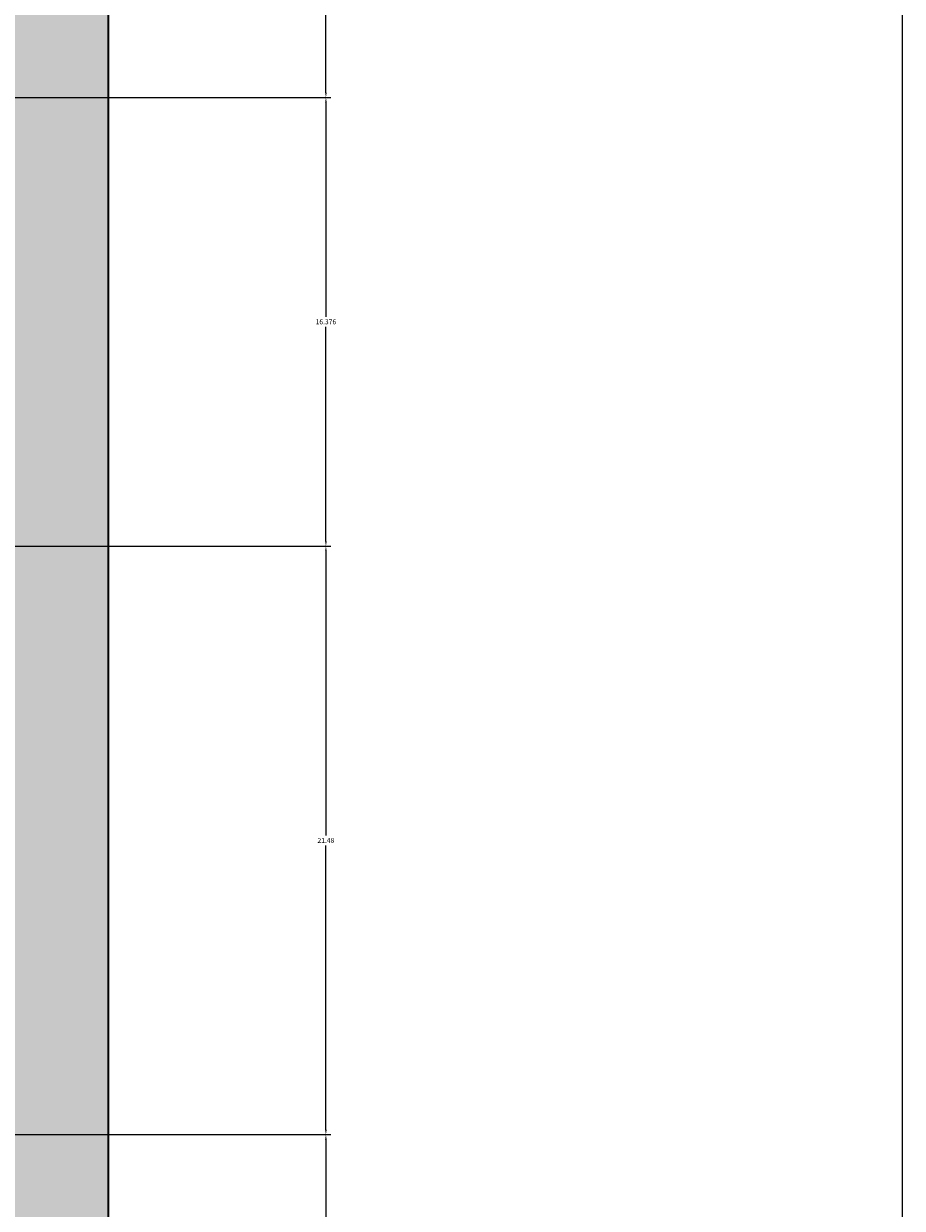
# Model space of a CAD drawing. Units: inches. Extents: x 4508 to 4723, y 847 to 1020.
# Tile 31 of 32: x 4691 to 4723, y 933 to 977. Entities that reach past the tile are written whole.
import ezdxf

# ---------------------------------------------------------------- set-up
doc = ezdxf.new("R2010")
doc.units = ezdxf.units.IN
for name, color, linetype, lineweight in [('A-ANNO-DIMS', 2, 'Continuous', 18), ('A-ANNO-TTLB', 7, 'Continuous', 25), ('A-WALL', 7, 'Continuous', 35), ('A-WALL-PATT', 254, 'Continuous', 13)]:
    doc.layers.add(name, color=color, linetype=linetype, lineweight=lineweight)
doc.styles.get("Standard").update_dxf_attribs({"font": 'arial.ttf'})
doc.dimstyles.get("Standard").update_dxf_attribs({"dimtxt": 0.18, "dimasz": 0.18, "dimexe": 0.18, "dimexo": 0.0625, "dimgap": 0.09, "dimtad": 0, "dimtih": 1, "dimtoh": 1, "dimdec": 4, "dimzin": 0, "dimdsep": 46, "dimtxsty": 'Standard', "dimcen": 0.09, "dimadec": 0, "dimazin": 0, "dimtfac": 1, "dimtdec": 4, "dimtofl": 0, "dimtmove": 0, "dimatfit": 3, "dimfxl": 1, "dimtolj": 1, "dimtzin": 0, "dimarcsym": 0})

# ---------------------------------------------------------------- blocks, each defined once
blk = doc.blocks.new('*D20')
at = {"layer": 'A-ANNO-DIMS', "color": 0, "lineweight": -2, "transparency": 16777216}
for p, q in [((4667.324, 936.122), (4702.124, 936.122)), ((4701.944, 935.942), (4701.944, 925.563)), ((4701.944, 914.821), (4701.944, 925.2)), ((4662.233, 914.641), (4702.124, 914.641))]:
    blk.add_line(p, q, dxfattribs=at)
at = {"layer": 'A-ANNO-DIMS', "color": 0, "lineweight": 9, "transparency": 16777216}
for points in [[(4701.914, 935.942), (4701.974, 935.942), (4701.944, 936.122)], [(4701.914, 914.821), (4701.974, 914.821), (4701.944, 914.641)]]:
    blk.add_solid(points, dxfattribs=at)
at = {"layer": 'Defpoints', "color": 0, "lineweight": 9, "transparency": 16777216}
for p in [(4667.262, 936.122), (4701.944, 936.122), (4662.171, 914.641)]:
    blk.add_point(p, dxfattribs=at)
at = {"layer": 'A-ANNO-DIMS', "color": 0, "transparency": 16777216, "insert": (4701.944, 925.381), "char_height": 0.18, "attachment_point": 5}
blk.add_mtext('\\A1;21.48', dxfattribs=at)
blk = doc.blocks.new('*D21')
at = {"layer": 'A-ANNO-DIMS', "color": 0, "lineweight": -2, "transparency": 16777216}
for p, q in [((4662.233, 957.602), (4702.124, 957.602)), ((4701.944, 957.422), (4701.944, 947.044)), ((4701.944, 936.302), (4701.944, 946.68)), ((4667.324, 936.122), (4702.124, 936.122))]:
    blk.add_line(p, q, dxfattribs=at)
at = {"layer": 'A-ANNO-DIMS', "color": 0, "lineweight": 9, "transparency": 16777216}
for points in [[(4701.914, 957.422), (4701.974, 957.422), (4701.944, 957.602)], [(4701.914, 936.302), (4701.974, 936.302), (4701.944, 936.122)]]:
    blk.add_solid(points, dxfattribs=at)
at = {"layer": 'Defpoints', "color": 0, "lineweight": 9, "transparency": 16777216}
for p in [(4662.171, 957.602), (4701.944, 957.602), (4667.262, 936.122)]:
    blk.add_point(p, dxfattribs=at)
at = {"layer": 'A-ANNO-DIMS', "color": 0, "transparency": 16777216, "insert": (4701.944, 946.862), "char_height": 0.18, "attachment_point": 5}
blk.add_mtext('\\A1;21.48', dxfattribs=at)
blk = doc.blocks.new('*D22')
at = {"layer": 'A-ANNO-DIMS', "color": 0, "lineweight": -2, "transparency": 16777216}
for p, q in [((4669.387, 973.978), (4702.124, 973.978)), ((4701.944, 973.798), (4701.944, 965.972)), ((4701.944, 957.782), (4701.944, 965.608)), ((4662.233, 957.602), (4702.124, 957.602))]:
    blk.add_line(p, q, dxfattribs=at)
at = {"layer": 'A-ANNO-DIMS', "color": 0, "lineweight": 9, "transparency": 16777216}
for points in [[(4701.914, 973.798), (4701.974, 973.798), (4701.944, 973.978)], [(4701.914, 957.782), (4701.974, 957.782), (4701.944, 957.602)]]:
    blk.add_solid(points, dxfattribs=at)
at = {"layer": 'Defpoints', "color": 0, "lineweight": 9, "transparency": 16777216}
for p in [(4669.325, 973.978), (4701.944, 973.978), (4662.171, 957.602)]:
    blk.add_point(p, dxfattribs=at)
at = {"layer": 'A-ANNO-DIMS', "color": 0, "transparency": 16777216, "insert": (4701.944, 965.79), "char_height": 0.18, "attachment_point": 5}
blk.add_mtext('\\A1;16.376', dxfattribs=at)
blk = doc.blocks.new('*D23')
at = {"layer": 'A-ANNO-DIMS', "color": 0, "lineweight": -2, "transparency": 16777216}
for p, q in [((4694.056, 994.747), (4702.124, 994.747)), ((4701.944, 994.567), (4701.944, 984.545)), ((4701.944, 974.158), (4701.944, 984.181)), ((4669.387, 973.978), (4702.124, 973.978))]:
    blk.add_line(p, q, dxfattribs=at)
at = {"layer": 'A-ANNO-DIMS', "color": 0, "lineweight": 9, "transparency": 16777216}
for points in [[(4701.914, 994.567), (4701.974, 994.567), (4701.944, 994.747)], [(4701.914, 974.158), (4701.974, 974.158), (4701.944, 973.978)]]:
    blk.add_solid(points, dxfattribs=at)
at = {"layer": 'Defpoints', "color": 0, "lineweight": 9, "transparency": 16777216}
for p in [(4693.994, 994.747), (4701.944, 994.747), (4669.325, 973.978)]:
    blk.add_point(p, dxfattribs=at)
at = {"layer": 'A-ANNO-DIMS', "color": 0, "transparency": 16777216, "insert": (4701.944, 984.363), "char_height": 0.18, "attachment_point": 5}
blk.add_mtext('\\A1;20.77', dxfattribs=at)

msp = doc.modelspace()

# ---------------------------------------------------------------- hatches: boundary and pattern name
at = {"layer": 'A-WALL-PATT', "transparency": 33554508}
h = msp.add_hatch(color=256, dxfattribs=at)
h.dxf.hatch_style = 1
h.paths.add_polyline_path([(4661.6706, 954.043, -0.3739004), (4658.5765, 957.6021, -1), (4665.7646, 957.6021, -0.3739004), (4662.6706, 954.043), (4662.6706, 944.4021, -0.2114781), (4670.3062, 945.0869), (4670.3062, 968.0592, -0.4632086), (4663.3246, 973.9783, -0.4632086), (4670.3062, 979.8975), (4670.3062, 994.7469), (4588.9938, 994.7469), (4588.9938, 904.7469), (4657.9938, 904.7469), (4657.9938, 886.7469), (4549.9938, 886.7469), (4549.9938, 878.7469), (4693.9938, 878.7469), (4693.9938, 994.7469), (4671.8062, 994.7469), (4671.8062, 979.4411, -0.2941682), (4675.3246, 973.9783, -0.2941682), (4671.8062, 968.5156), (4671.8062, 944.4278, -0.2741114), (4676.7298, 936.1217, -0.2741114), (4671.8062, 927.8155), (4671.8062, 907.6998, -0.3779645), (4677.0562, 901.7469, -0.3779645), (4671.8062, 895.7939), (4671.8062, 883.7469), (4670.3062, 883.7469), (4670.3062, 895.7939, -0.3779645), (4665.0562, 901.7469, -0.3779645), (4670.3062, 907.6998), (4670.3062, 927.1564, -0.2114781), (4662.6706, 927.8412), (4662.6706, 918.2003, -0.3739004), (4665.7646, 914.6412, -1), (4658.5765, 914.6412, -0.3739004), (4661.6706, 918.2003), (4661.6706, 928.4807, -0.2391825), (4657.7936, 936.1217, -0.2391825), (4661.6706, 943.7626)])

# ---------------------------------------------------------------- linework, layer by layer
at = {"layer": 'A-ANNO-TTLB'}
msp.add_lwpolyline([(4508.3867, 1019.9118), (4722.9774, 1019.9118), (4722.9774, 846.9535), (4508.3867, 846.9535)], close=True, dxfattribs=at)
at = {"layer": 'A-WALL'}
msp.add_line((4693.9938, 994.7469), (4693.9938, 874.7469), dxfattribs=at)

# ---------------------------------------------------------------- dimensions: what is measured, and where the dimension line sits
at = {"layer": 'A-ANNO-DIMS'}
for base, p1, p2, override, picture, middle in [((4701.9438, 994.7469), (4669.3246, 973.9783), (4693.9938, 994.7469), {"dimdec": 2, "dimlfac": 1, "dimrnd": 0, "dimzin": 0, "dimdsep": 46, "dimlunit": 2}, '*D23', (4701.9438, 984.3626)), ((4701.9438, 973.9783), (4662.1706, 957.6021), (4669.3246, 973.9783), {"dimdec": 3, "dimlfac": 1, "dimrnd": 0, "dimzin": 0, "dimdsep": 46, "dimlunit": 2}, '*D22', (4701.9438, 965.7902)), ((4701.9438, 957.6021), (4667.2617, 936.1217), (4662.1706, 957.6021), {"dimdec": 2, "dimlfac": 1, "dimrnd": 0, "dimzin": 0, "dimdsep": 46, "dimlunit": 2}, '*D21', (4701.9438, 946.8619)), ((4701.9438, 936.1217), (4662.1706, 914.6412), (4667.2617, 936.1217), {"dimdec": 2, "dimlfac": 1, "dimrnd": 0, "dimzin": 0, "dimdsep": 46, "dimlunit": 2}, '*D20', (4701.9438, 925.3814))]:
    dim = msp.add_linear_dim(base=base, p1=p1, p2=p2, angle=90, dimstyle='Standard', override=override, dxfattribs=at)
    dim.commit()
    dim.dimension.update_dxf_attribs({"geometry": picture, "text_midpoint": middle})

doc.saveas('drawing.dxf')
